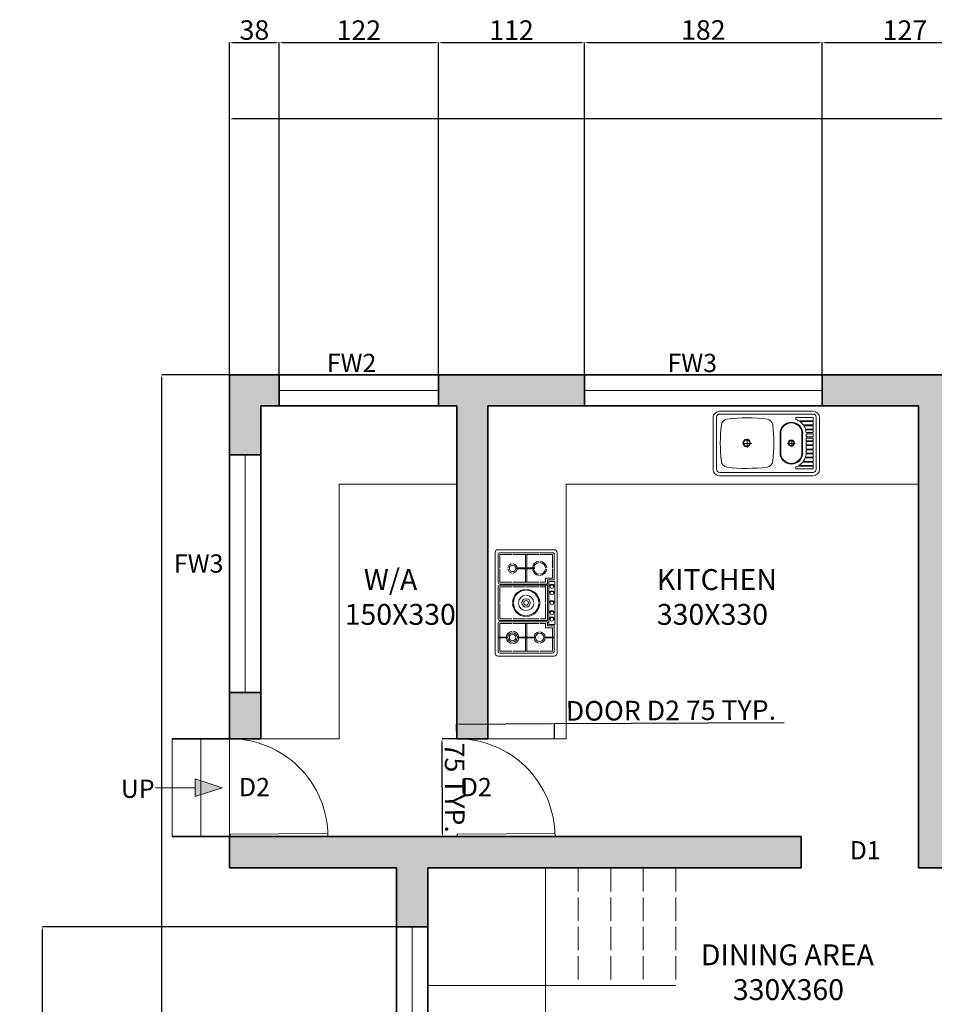
# Model space of a CAD drawing. Units: centimetres. Extents: x 2449 to 7478, y 778 to 2486.
# Tile 8 of 9: x 5994 to 6695, y 1732 to 2486. Entities that reach past the tile are written whole.
import ezdxf

# ---------------------------------------------------------------- set-up
doc = ezdxf.new("R2010")
doc.units = ezdxf.units.CM
doc.linetypes.add('ACAD_ISO02W100', pattern=[15, 12, -3])
for name, color, linetype, lineweight in [('A-ANNO-DIMS', 2, 'Continuous', 18), ('A-ANNO-SYMB', 8, 'Continuous', 18), ('A-ANNO-TEXT', 7, 'Continuous', 18), ('A-AREA-IDEN', 7, 'Continuous', 18), ('A-DOOR', 4, 'Continuous', 18), ('A-EQPM', 8, 'Continuous', 18), ('A-FLOR-CASE', 8, 'Continuous', 18), ('A-FLOR-FIXT', 8, 'Continuous', 18), ('A-FLOR-STRS', 7, 'Continuous', 18), ('A-FLOR-STRS-OVHD', 7, 'ACAD_ISO02W100', 13), ('A-WALL', 7, 'Continuous', 35), ('A-WALL-PATT', 7, 'Continuous', 13), ('Win', 1, 'Continuous', 18)]:
    doc.layers.add(name, color=color, linetype=linetype, lineweight=lineweight)
doc.styles.get("Standard").update_dxf_attribs({"font": 'arial.ttf'})
doc.dimstyles.new('ISO-25', dxfattribs={"dimtxt": 15, "dimasz": 2.5, "dimexe": 0, "dimexo": 0, "dimgap": 0, "dimtad": 1, "dimtxsty": 'Standard', "dimcen": 2.5, "dimadec": 0, "dimazin": 0, "dimtfac": 1, "dimtmove": 0, "dimatfit": 3, "dimfxl": 1, "dimarcsym": 0})

# ---------------------------------------------------------------- blocks, each defined once
blk = doc.blocks.new('sink 1')
for points in [[(-7.34, 1.48), (-7.34, 22.73)], [(-6.56, 1.48), (-6.56, 22.73)], [(5.86, 24.22), (-5.86, 24.22)], [(6.01, 23.43), (-5.86, 23.43)], [(6.72, 1.48), (6.72, 22.73)], [(7.34, 1.48), (7.34, 22.73)], [(1.09, 16.48), (-0.94, 16.48)], [(0, 15.39), (0, 17.42)], [(-2.09, 8.99), (2.28, 8.99)], [(-2.09, 8.84), (2.28, 8.84)], [(0, 5.55), (0, 7.26)], [(-5.78, 5.39), (-5.78, 5.39)], [(-5.31, 5.39), (-5.31, 5.39)], [(-5.16, 4.92), (-5.16, 4.92)], [(-5, 1.48), (-5, 4.69)], [(0.78, 6.33), (-0.78, 6.33)], [(5.16, 4.92), (5.16, 4.92)], [(5.94, 5.39), (5.94, 5.39)], [(-5, 1.48), (-4.22, 1.48), (-4.22, 3.83)], [(-4.84, 4.45), (-4.84, 4.45)], [(-4.22, 3.83), (-4.22, 3.83)], [(-4.06, 1.48), (-4.06, 3.69)], [(-4.06, 1.48), (-3.28, 1.48), (-3.28, 3.27)], [(-3.91, 3.52), (-3.91, 3.52)], [(-3.28, 3.2), (-3.28, 3.2)], [(-3.12, 3.2), (-3.12, 3.2)], [(-2.34, 3.05), (-2.34, 3.05)], [(-2.19, 3.05), (-2.19, 3.05)], [(-2.09, 3.99), (2.28, 3.99)], [(-2.09, 3.84), (2.28, 3.84)], [(-1.41, 3.05), (-1.41, 3.05)], [(-1.25, 3.05), (-1.25, 3.05)], [(-0.47, 1.48), (-1.25, 1.48), (-1.25, 3.05), (-0.47, 3.05)], [(-0.62, 3.05), (-0.62, 3.05)], [(-0.47, 1.48), (-0.47, 3.05)], [(-0.31, 3.05), (-0.31, 3.05)], [(0.47, 1.48), (-0.31, 1.48), (-0.31, 3.05), (0.47, 3.05)], [(0.31, 3.05), (0.31, 3.05)], [(0.47, 1.48), (0.47, 3.05)], [(0.62, 3.05), (0.62, 3.05)], [(1.25, 3.05), (1.25, 3.05)], [(1.56, 3.05), (1.56, 3.05)], [(2.19, 3.05), (2.19, 3.05)], [(2.5, 3.05), (2.5, 3.05)], [(3.12, 3.2), (3.12, 3.2)], [(3.28, 1.48), (4.06, 1.48), (4.06, 3.57)], [(3.28, 1.48), (3.28, 3.2)], [(3.44, 3.2), (3.44, 3.2)], [(4.06, 3.52), (4.06, 3.52)], [(4.22, 1.48), (4.22, 3.67)], [(4.37, 3.83), (4.37, 3.83)], [(5, 4.45), (5, 4.45)], [(6.01, 0.78), (-5.86, 0.78)], [(5.86, 0), (-5.86, 0)], [(-5.78, 1.48), (-5.78, 1.48)], [(-5.16, 1.48), (-5.16, 1.48)], [(-4.84, 1.48), (-4.84, 1.48)], [(-4.22, 1.48), (-4.22, 1.48)], [(-3.91, 1.48), (-3.91, 1.48)], [(-3.28, 1.48), (-3.28, 1.48)], [(-3.12, 1.48), (-3.12, 1.48)], [(-2.34, 1.48), (-2.34, 1.48)], [(-2.19, 1.48), (-2.19, 1.48)], [(-1.41, 1.48), (-1.41, 1.48)], [(-1.25, 1.48), (-1.25, 1.48)], [(-0.62, 1.48), (-0.62, 1.48)], [(-0.31, 1.48), (-0.31, 1.48)], [(0.31, 1.48), (0.31, 1.48)], [(0.62, 1.48), (0.62, 1.48)], [(1.25, 1.48), (1.25, 1.48)], [(1.56, 1.48), (1.56, 1.48)], [(2.19, 1.48), (2.19, 1.48)], [(2.5, 1.48), (2.5, 1.48)], [(3.12, 1.48), (3.12, 1.48)], [(3.44, 1.48), (3.44, 1.48)], [(4.06, 1.48), (4.06, 1.48)], [(4.37, 1.48), (4.37, 1.48)], [(5, 1.48), (5, 1.48)], [(5.16, 1.48), (5.16, 1.48)], [(5.94, 1.48), (5.94, 1.48)]]:
    blk.add_lwpolyline(points)
for points in [[(-5.16, 4.92), (-5.16, 1.48), (-5.78, 1.48), (-5.78, 5.39), (-5.31, 5.39, -0.068511), (-5.16, 4.92)], [(5.16, 4.92, 0.248301), (5.47, 5.39), (5.94, 5.39), (5.94, 1.48), (5.16, 1.48), (5.16, 4.92)], [(4.06, 3.57, -0.061679), (3.32, 3.22)], [(4.22, 1.48), (5, 1.48), (5, 4.45, -0.083542), (4.22, 3.67, -0.083542)]]:
    blk.add_lwpolyline(points, format="xyb")
for points in [[(-3.12, 3.22), (-3.12, 1.48), (-2.34, 1.48), (-2.34, 3.05, -0.06228)], [(2.5, 3.05), (2.5, 1.48), (3.12, 1.48), (3.12, 3.2, -0.050256)]]:
    blk.add_lwpolyline(points, format="xyb", close=True)
for points in [[(-2.19, 3.05), (-1.41, 3.05), (-1.41, 1.48), (-2.19, 1.48)], [(0.62, 3.05), (1.25, 3.05), (1.25, 1.48), (0.62, 1.48)], [(2.19, 1.48), (2.19, 3.05), (1.56, 3.05), (1.56, 1.48)]]:
    blk.add_lwpolyline(points, close=True)
for centre, radius in [((0.09, 16.57), 0.859), ((0.09, 16.57), 0.703), ((0.09, 6.41), 0.703), ((0.09, 6.41), 0.547)]:
    blk.add_circle(centre, radius)
for centre, radius, start, end in [((-5.86, 22.73), 1.48, 90, 180), ((-5.86, 22.73), 0.703, 90, 180), ((0.09, -12.65), 35.23, 83.2159, 96.7841), ((5.86, 22.73), 1.48, 360, 90), ((6.01, 22.73), 0.703, 0, 90), ((30.19, 16.56), 35.85, 172.7947, 187.4213), ((-3.87, 20.82), 1.53, 97.3256, 171.1849), ((4.06, 20.82), 1.53, 8.8151, 82.6744), ((-30, 16.56), 35.85, 352.5787, 7.2053), ((-3.89, 12.12), 1.48, 187.4212, 263.2159), ((4.08, 12.12), 1.48, 276.7841, 352.5788), ((-2.1, 6.41), 2.58, 90, 270), ((0.09, 45.63), 35.23, 263.2159, 276.7841), ((2.28, 6.41), 2.58, 270, 90), ((-2.1, 6.41), 2.42, 90, 270), ((2.28, 6.41), 2.42, 270, 90), ((-2.15, 6.48), 3.36, 212.1095, 232.0862), ((-2.1, 6.41), 3.36, 234.156, 249.3275), ((2.14, 6.36), 3.36, 289.8633, 290.5971), ((-5.86, 1.48), 1.48, 180, 270), ((-5.86, 1.48), 0.703, 180, 270), ((5.86, 1.48), 1.48, 270, 0), ((6.01, 1.48), 0.703, 270, 360)]:
    blk.add_arc(centre, radius, start, end)
blk = doc.blocks.new('STOVE')
for p, q in [((11.85, 19.7), (11.55, 19.7)), ((11.55, 16.92), (11.55, 19.7)), ((11.85, 16.92), (11.55, 16.92)), ((11.85, 16.92), (11.85, 19.7)), ((-11.85, 13.73), (-11.85, 7.62)), ((-11.85, 13.73), (-11.55, 13.73)), ((-11.55, 13.73), (-11.55, 7.62)), ((-11.85, 10.75), (-16.4, 10.75)), ((-11.85, 10.25), (-16.4, 10.25)), ((-7, 10.75), (-11.55, 10.75)), ((-7, 10.25), (-11.55, 10.25)), ((7, 10.75), (11.55, 10.75)), ((7, 10.25), (11.55, 10.25)), ((11.85, 13.23), (11.55, 13.23)), ((11.55, 13.23), (11.55, 7.57)), ((11.85, 13.23), (11.85, 7.57)), ((11.85, 10.75), (16.4, 10.75)), ((11.85, 10.25), (16.4, 10.25)), ((-11.85, 7.62), (-11.55, 7.62)), ((11.85, 7.57), (11.55, 7.57)), ((-7, 3.9), (-8.4, 3.9)), ((-5.4, 3.9), (-6, 3.9)), ((-5.4, 3.9), (-0.15, 3.9)), ((0.15, 3.9), (5.4, 3.9)), ((7, 3.9), (8.4, 3.9)), ((8.4, 3.9), (8.4, 1.6)), ((11.85, 4.28), (11.55, 4.28)), ((11.55, 4.28), (11.55, 1.3)), ((11.85, 4.28), (11.85, 1.3)), ((-7.8, 3.3), (-7.8, 1)), ((-6.4, 3.3), (-7.8, 3.3)), ((7.3, 2.8), (-7.3, 2.8)), ((-7.3, 2.8), (-7.3, 0.8)), ((7.3, 0.8), (-7.3, 0.8)), ((6.4, 3.3), (7.8, 3.3)), ((7.3, 2.8), (7.3, 0.8)), ((7.8, 3.3), (7.8, 1)), ((11.85, 1.3), (11.55, 1.3))]:
    blk.add_line(p, q)
for points in [[(-17, 21), (17, 21, -0.414214), (18, 20), (18, 1, -0.414214), (17, 0), (-17, 0, -0.414214), (-18, 1), (-18, 20, -0.414214)], [(6, 3.3), (-6, 3.3), (-6, 19.4, -0.414214), (-5.4, 20), (5.4, 20, -0.414214), (6, 19.4)]]:
    blk.add_lwpolyline(points, format="xyb", close=True)
for points in [[(-7.8, 1), (-16.4, 1, -0.414214), (-17, 1.6), (-17, 19.4, -0.414214), (-16.4, 20), (-7, 20, -0.414214), (-6.4, 19.4), (-6.4, 3.3)], [(6.4, 19.4, -0.414214), (7, 20), (16.4, 20, -0.414214), (17, 19.4), (17, 1.6, -0.414214), (16.4, 1), (7.8, 1)]]:
    blk.add_lwpolyline(points, format="xyb")
for points in [[(-16.4, 15.22), (-16.4, 19.4), (-11.85, 19.4)], [(-11.55, 19.4), (-7, 19.4), (-7, 15.22)], [(-5.4, 15.22), (-5.4, 19.4), (-0.15, 19.4)], [(0.15, 19.4), (5.4, 19.4), (5.4, 15.22)], [(6.4, 3.3), (6.4, 19.4)], [(7, 15.22), (7, 19.4), (11.55, 19.4)], [(11.85, 19.4), (16.4, 19.4), (16.4, 15.22)], [(-16.4, 6.08), (-16.4, 14.92)], [(-7, 14.92), (-7, 6.08)], [(-5.4, 10.65), (-5.4, 14.92)], [(5.4, 14.92), (5.4, 10.65)], [(7, 6.08), (7, 14.92)], [(16.4, 14.92), (16.4, 6.08)], [(-5.4, 6.08), (-5.4, 10.35)], [(5.4, 10.35), (5.4, 6.08)], [(-11.85, 1.6), (-16.4, 1.6), (-16.4, 5.77)], [(-8.4, 3.9), (-8.4, 1.6), (-11.55, 1.6)], [(-7, 5.77), (-7, 3.9)], [(-5.4, 3.9), (-5.4, 5.77)], [(5.4, 5.77), (5.4, 3.9)], [(7, 3.9), (7, 5.77)], [(16.4, 5.77), (16.4, 1.6), (11.85, 1.6)], [(11.55, 1.6), (8.4, 1.6)]]:
    blk.add_lwpolyline(points)
for centre, radius in [((-11.7, 15.07), 1.1), ((11.7, 15.07), 1.6), ((11.7, 15.07), 1.1), ((0, 10.5), 1.4), ((0, 10.5), 0.8), ((11.7, 5.93), 1.4), ((-5.49, 1.8), 0.6), ((-3.3, 1.8), 0.6), ((0, 1.8), 0.6), ((3.39, 1.8), 0.6), ((5.57, 1.8), 0.6)]:
    blk.add_circle(centre, radius)
for centre, radius, start, end in [((11.7, 15.07), 2.1, 94.096, 175.904), ((11.7, 15.07), 2.1, 4.096, 85.904), ((-11.7, 15.07), 1.6, 95.3794, 174.6206), ((-11.7, 15.07), 1.6, 185.3794, 264.6206), ((-11.7, 15.07), 1.6, 5.3794, 84.6206), ((-11.7, 15.07), 1.6, 275.3794, 354.6206), ((0, 10.5), 4.6, 91.8687, 178.1313), ((0, 10.5), 4.3, 91.9991, 178.0009), ((0, 10.5), 4.6, 1.8687, 88.1313), ((0, 10.5), 4.3, 1.9991, 88.0009), ((11.7, 15.07), 2.1, 184.096, 265.904), ((11.7, 15.07), 2.1, 274.096, 355.904), ((0, 10.5), 4.6, 181.8687, 268.1313), ((0, 10.5), 4.3, 181.9991, 268.0009), ((0, 10.5), 2.6, 93.3074, 176.6926), ((0, 10.5), 2.6, 183.3074, 266.6926), ((0, 10.5), 2.6, 3.3074, 86.6926), ((0, 10.5), 4.6, 271.8687, 358.1313), ((0, 10.5), 4.3, 271.9991, 358.0009), ((0, 10.5), 2.6, 273.3074, 356.6926), ((-11.7, 5.93), 2.4, 93.5833, 176.4167), ((-11.7, 5.93), 2, 94.3012, 175.6988), ((-11.7, 5.93), 2.4, 3.5833, 86.4167), ((-11.7, 5.93), 2, 4.3012, 85.6988), ((11.7, 5.93), 1.9, 94.5281, 175.4719), ((11.7, 5.93), 1.9, 4.5281, 85.4719), ((-11.7, 5.93), 2.4, 183.5833, 266.4167), ((-11.7, 5.93), 2, 184.3012, 265.6988), ((-11.7, 5.93), 2.4, 273.5833, 356.4167), ((-11.7, 5.93), 2, 274.3012, 355.6988), ((11.7, 5.93), 1.9, 184.5281, 265.4719), ((11.7, 5.93), 1.9, 274.5281, 355.4719), ((-5.49, 1.8), 0.846, 89.9979, 270), ((-3.3, 1.8), 0.846, 89.9979, 270), ((0, 1.8), 0.846, 89.9979, 270), ((3.39, 1.8), 0.846, 89.9979, 270), ((5.57, 1.8), 0.846, 89.9979, 270)]:
    blk.add_arc(centre, radius, start, end)
blk = doc.blocks.new('3')
for p, q in [((5936.31, 1821.57), (5936.31, 1746.57)), ((5938.31, 1821.57), (5938.31, 1746.57)), ((5938.31, 1746.57), (5936.31, 1746.57))]:
    blk.add_line(p, q)
blk.add_arc((5936.31, 1746.57), 75, 0, 90)
blk = doc.blocks.new('*D63')
at = {"layer": 'A-ANNO-DIMS', "color": 0, "lineweight": -2, "transparency": 16777216}
for p, q in [((6155.01, 2214.34), (6155.01, 2410.3)), ((7386.51, 2410.3), (6157.51, 2410.3)), ((7389.01, 2382.34), (7389.01, 2410.3))]:
    blk.add_line(p, q, dxfattribs=at)
at = {"layer": 'A-ANNO-DIMS', "color": 0, "transparency": 16777216}
for points in [[(6157.51, 2410.71), (6157.51, 2409.88), (6155.01, 2410.3)], [(7386.51, 2410.71), (7386.51, 2409.88), (7389.01, 2410.3)]]:
    blk.add_solid(points, dxfattribs=at)
at = {"layer": 'Defpoints', "color": 0, "transparency": 16777216}
for p in [(6155.01, 2410.3), (7389.01, 2382.34), (6155.01, 2214.34)]:
    blk.add_point(p, dxfattribs=at)
at = {"layer": 'A-ANNO-DIMS', "color": 0, "transparency": 16777216, "insert": (6772.01, 2417.96), "char_height": 15, "attachment_point": 5}
blk.add_mtext('1234', dxfattribs=at)
blk = doc.blocks.new('*D66')
at = {"layer": 'A-ANNO-DIMS', "color": 0, "lineweight": -2, "transparency": 16777216}
for p, q in [((6155.01, 2214.34), (6103.02, 2214.34)), ((6103.02, 1070.84), (6103.02, 2211.84)), ((6283.01, 1068.34), (6103.02, 1068.34))]:
    blk.add_line(p, q, dxfattribs=at)
at = {"layer": 'A-ANNO-DIMS', "color": 0, "transparency": 16777216}
for points in [[(6102.61, 2211.84), (6103.44, 2211.84), (6103.02, 2214.34)], [(6102.61, 1070.84), (6103.44, 1070.84), (6103.02, 1068.34)]]:
    blk.add_solid(points, dxfattribs=at)
at = {"layer": 'Defpoints', "color": 0, "transparency": 16777216}
for p in [(6103.02, 2214.34), (6155.01, 2214.34), (6283.01, 1068.34)]:
    blk.add_point(p, dxfattribs=at)
at = {"layer": 'A-ANNO-DIMS', "color": 0, "transparency": 16777216, "insert": (6095.36, 1641.34), "char_height": 15, "attachment_point": 5, "rotation": 90}
blk.add_mtext('1146', dxfattribs=at)
blk = doc.blocks.new('COUNTER-KITCHEN')
for p, q in [((0, 0), (270, 0)), ((0, 0), (0, -195)), ((0, -195), (-60, -195))]:
    blk.add_line(p, q)
blk = doc.blocks.new('COUNTER-UTILITY')
for p, q in [((0, 0), (90, 0)), ((0, 0), (0, -195)), ((-60, -195), (0, -195))]:
    blk.add_line(p, q)
blk = doc.blocks.new('ARROW-ENTRY-UP')
at = {"transparency": 33554687}
h = blk.add_hatch(color=256, dxfattribs=at)
h.dxf.hatch_style = 1
h.paths.add_polyline_path([(-6.84, 30.34), (6.84, 30.34), (0, 51.25)])
blk.add_line((0, 30.34), (0, 0))
blk.add_lwpolyline([(0, 51.25), (-6.84, 30.34), (6.84, 30.34)], close=True)
blk = doc.blocks.new('*D76')
at = {"layer": 'A-ANNO-DIMS', "color": 0, "lineweight": -2, "transparency": 16777216}
for p, q in [((6329.01, 1935.34), (6328.95, 1946.59)), ((6331.45, 1946.6), (6401.45, 1946.93)), ((6403.95, 1946.94), (6580.01, 1947.78)), ((6404.01, 1935.69), (6403.95, 1946.94))]:
    blk.add_line(p, q, dxfattribs=at)
at = {"layer": 'A-ANNO-DIMS', "color": 0, "transparency": 16777216}
for points in [[(6331.45, 1947.02), (6331.45, 1946.18), (6328.95, 1946.59)], [(6401.45, 1947.35), (6401.45, 1946.52), (6403.95, 1946.94)]]:
    blk.add_solid(points, dxfattribs=at)
at = {"layer": 'Defpoints', "color": 0, "transparency": 16777216}
for p in [(6403.95, 1946.94), (6329.01, 1935.34), (6404.01, 1935.69)]:
    blk.add_point(p, dxfattribs=at)
at = {"layer": 'A-ANNO-DIMS', "color": 0, "transparency": 16777216, "insert": (6493.2, 1955.13), "char_height": 15, "attachment_point": 5, "rotation": 0.27085}
blk.add_mtext('DOOR D2 75 TYP.', dxfattribs=at)
blk = doc.blocks.new('*D77')
at = {"layer": 'A-ANNO-DIMS', "color": 0, "lineweight": -2, "transparency": 16777216}
for p, q in [((6329.01, 1935.34), (6317.76, 1935.29)), ((6318.1, 1862.79), (6317.77, 1932.79)), ((6329.36, 1860.34), (6318.11, 1860.29))]:
    blk.add_line(p, q, dxfattribs=at)
at = {"layer": 'A-ANNO-DIMS', "color": 0, "transparency": 16777216}
for points in [[(6318.18, 1932.79), (6317.35, 1932.78), (6317.76, 1935.29)], [(6318.52, 1862.79), (6317.68, 1862.79), (6318.11, 1860.29)]]:
    blk.add_solid(points, dxfattribs=at)
at = {"layer": 'Defpoints', "color": 0, "transparency": 16777216}
for p in [(6317.76, 1935.29), (6329.01, 1935.34), (6329.36, 1860.34)]:
    blk.add_point(p, dxfattribs=at)
at = {"layer": 'A-ANNO-DIMS', "color": 0, "transparency": 16777216, "insert": (6325.56, 1897.82), "char_height": 15, "attachment_point": 5, "rotation": 270.27085}
blk.add_mtext('75 TYP.', dxfattribs=at)
blk = doc.blocks.new('*D105')
at = {"layer": 'A-ANNO-DIMS', "color": 0, "lineweight": -2, "transparency": 16777216}
for p, q in [((6155.01, 2214.34), (6155.01, 2468.84)), ((6157.51, 2468.84), (6190.51, 2468.84)), ((6193.01, 2214.34), (6193.01, 2468.84))]:
    blk.add_line(p, q, dxfattribs=at)
at = {"layer": 'A-ANNO-DIMS', "color": 0, "transparency": 16777216}
for points in [[(6157.51, 2469.26), (6157.51, 2468.42), (6155.01, 2468.84)], [(6190.51, 2469.26), (6190.51, 2468.42), (6193.01, 2468.84)]]:
    blk.add_solid(points, dxfattribs=at)
at = {"layer": 'Defpoints', "color": 0, "transparency": 16777216}
for p in [(6193.01, 2468.84), (6155.01, 2214.34), (6193.01, 2214.34)]:
    blk.add_point(p, dxfattribs=at)
at = {"layer": 'A-ANNO-DIMS', "color": 0, "transparency": 16777216, "insert": (6174.01, 2476.5), "char_height": 15, "attachment_point": 5}
blk.add_mtext('38', dxfattribs=at)
blk = doc.blocks.new('*D106')
at = {"layer": 'A-ANNO-DIMS', "color": 0, "lineweight": -2, "transparency": 16777216}
for p, q in [((6193.01, 2214.34), (6193.01, 2468.84)), ((6195.51, 2468.84), (6312.51, 2468.84)), ((6315.01, 2214.34), (6315.01, 2468.84))]:
    blk.add_line(p, q, dxfattribs=at)
at = {"layer": 'A-ANNO-DIMS', "color": 0, "transparency": 16777216}
for points in [[(6195.51, 2469.26), (6195.51, 2468.42), (6193.01, 2468.84)], [(6312.51, 2469.26), (6312.51, 2468.42), (6315.01, 2468.84)]]:
    blk.add_solid(points, dxfattribs=at)
at = {"layer": 'Defpoints', "color": 0, "transparency": 16777216}
for p in [(6315.01, 2468.84), (6193.01, 2214.34), (6315.01, 2214.34)]:
    blk.add_point(p, dxfattribs=at)
at = {"layer": 'A-ANNO-DIMS', "color": 0, "transparency": 16777216, "insert": (6254.01, 2476.37), "char_height": 15, "attachment_point": 5}
blk.add_mtext('122', dxfattribs=at)
blk = doc.blocks.new('*D107')
at = {"layer": 'A-ANNO-DIMS', "color": 0, "lineweight": -2, "transparency": 16777216}
for p, q in [((6315.01, 2214.34), (6315.01, 2468.84)), ((6317.51, 2468.84), (6424.51, 2468.84)), ((6427.01, 2214.34), (6427.01, 2468.84))]:
    blk.add_line(p, q, dxfattribs=at)
at = {"layer": 'A-ANNO-DIMS', "color": 0, "transparency": 16777216}
for points in [[(6317.51, 2469.26), (6317.51, 2468.42), (6315.01, 2468.84)], [(6424.51, 2469.26), (6424.51, 2468.42), (6427.01, 2468.84)]]:
    blk.add_solid(points, dxfattribs=at)
at = {"layer": 'Defpoints', "color": 0, "transparency": 16777216}
for p in [(6427.01, 2468.84), (6315.01, 2214.34), (6427.01, 2214.34)]:
    blk.add_point(p, dxfattribs=at)
at = {"layer": 'A-ANNO-DIMS', "color": 0, "transparency": 16777216, "insert": (6371.01, 2476.37), "char_height": 15, "attachment_point": 5}
blk.add_mtext('112', dxfattribs=at)
blk = doc.blocks.new('*D108')
at = {"layer": 'A-ANNO-DIMS', "color": 0, "lineweight": -2, "transparency": 16777216}
for p, q in [((6427.01, 2214.34), (6427.01, 2468.84)), ((6429.51, 2468.84), (6606.51, 2468.84)), ((6609.01, 2214.34), (6609.01, 2468.84))]:
    blk.add_line(p, q, dxfattribs=at)
at = {"layer": 'A-ANNO-DIMS', "color": 0, "transparency": 16777216}
for points in [[(6429.51, 2469.26), (6429.51, 2468.42), (6427.01, 2468.84)], [(6606.51, 2469.26), (6606.51, 2468.42), (6609.01, 2468.84)]]:
    blk.add_solid(points, dxfattribs=at)
at = {"layer": 'Defpoints', "color": 0, "transparency": 16777216}
for p in [(6609.01, 2468.84), (6427.01, 2214.34), (6609.01, 2214.34)]:
    blk.add_point(p, dxfattribs=at)
at = {"layer": 'A-ANNO-DIMS', "color": 0, "transparency": 16777216, "insert": (6518.01, 2476.5), "char_height": 15, "attachment_point": 5}
blk.add_mtext('182', dxfattribs=at)
blk = doc.blocks.new('*D109')
at = {"layer": 'A-ANNO-DIMS', "color": 0, "lineweight": -2, "transparency": 16777216}
for p, q in [((6609.01, 2214.34), (6609.01, 2468.84)), ((6611.51, 2468.84), (6733.51, 2468.84)), ((6736.01, 2214.34), (6736.01, 2468.84))]:
    blk.add_line(p, q, dxfattribs=at)
at = {"layer": 'A-ANNO-DIMS', "color": 0, "transparency": 16777216}
for points in [[(6611.51, 2469.26), (6611.51, 2468.42), (6609.01, 2468.84)], [(6733.51, 2469.26), (6733.51, 2468.42), (6736.01, 2468.84)]]:
    blk.add_solid(points, dxfattribs=at)
at = {"layer": 'Defpoints', "color": 0, "transparency": 16777216}
for p in [(6736.01, 2468.84), (6609.01, 2214.34), (6736.01, 2214.34)]:
    blk.add_point(p, dxfattribs=at)
at = {"layer": 'A-ANNO-DIMS', "color": 0, "transparency": 16777216, "insert": (6672.51, 2476.37), "char_height": 15, "attachment_point": 5}
blk.add_mtext('127', dxfattribs=at)
blk = doc.blocks.new('*D115')
at = {"layer": 'A-ANNO-DIMS', "color": 0, "lineweight": -2, "transparency": 16777216}
for p, q in [((6283.01, 1791.34), (6011.65, 1791.34)), ((6011.65, 1553.84), (6011.65, 1788.84)), ((6283.01, 1551.34), (6011.65, 1551.34))]:
    blk.add_line(p, q, dxfattribs=at)
at = {"layer": 'A-ANNO-DIMS', "color": 0, "transparency": 16777216}
for points in [[(6011.23, 1788.84), (6012.07, 1788.84), (6011.65, 1791.34)], [(6011.23, 1553.84), (6012.07, 1553.84), (6011.65, 1551.34)]]:
    blk.add_solid(points, dxfattribs=at)
at = {"layer": 'Defpoints', "color": 0, "transparency": 16777216}
for p in [(6011.65, 1791.34), (6283.01, 1791.34), (6283.01, 1551.34)]:
    blk.add_point(p, dxfattribs=at)
at = {"layer": 'A-ANNO-DIMS', "color": 0, "transparency": 16777216, "insert": (6003.99, 1671.34), "char_height": 15, "attachment_point": 5, "rotation": 90}
blk.add_mtext('240', dxfattribs=at)

msp = doc.modelspace()

# ---------------------------------------------------------------- hatches: boundary and pattern name
at = {"layer": 'A-WALL-PATT'}
h = msp.add_hatch(color=256, dxfattribs=at)
h.dxf.hatch_style = 1
h.paths.add_polyline_path([(6637.006, 1092.34), (6563.006, 1092.34), (6563.006, 1068.34), (6661.006, 1068.34), (6661.006, 1476.34), (6637.006, 1476.34)])
h.paths.add_polyline_path([(6283.006, 1167.34), (6307.006, 1167.34), (6307.006, 1377.34), (6283.006, 1377.34)])
h.paths.add_polyline_path([(6381.006, 1068.34), (6381.006, 1092.34), (6307.006, 1092.34), (6307.006, 1112.34), (6283.006, 1112.34), (6283.006, 1068.34)])
h.paths.add_polyline_path([(6307.006, 1551.34), (6283.006, 1551.34), (6283.006, 1432.34), (6307.006, 1432.34), (6307.006, 1452.34), (6547.006, 1452.34), (6547.006, 1476.34), (6307.006, 1476.34)])
h.paths.add_polyline_path([(7011.006, 1654.34), (7011.006, 1266.34), (6982.006, 1266.34), (6982.006, 1242.34), (7035.006, 1242.34), (7035.006, 1404.34), (7059.006, 1404.34), (7059.006, 1428.34), (7035.006, 1428.34), (7035.006, 1678.34), (6837.006, 1678.34), (6837.006, 1654.34)])
h.paths.add_polyline_path([(6800.006, 1266.34), (6771.006, 1266.34), (6771.006, 1242.34), (6800.006, 1242.34)])
h.paths.add_polyline_path([(7389.006, 1506.339), (7365.006, 1506.339), (7365.006, 1428.34), (7341.006, 1428.34), (7341.006, 1404.34), (7389.006, 1404.34)])
h.paths.add_polyline_path([(7286.006, 1404.34), (7286.006, 1428.34), (7114.006, 1428.34), (7114.006, 1404.34)])
h.paths.add_polyline_path([(7365.006, 1688.339), (7389.006, 1688.339), (7389.006, 1826.34), (7365.006, 1826.34), (7365.006, 1792.34), (7224.006, 1792.34), (7224.006, 1768.34), (7365.006, 1768.34)])
h.paths.add_polyline_path([(7365.006, 1956.34), (7125.006, 1956.34), (7125.006, 1792.34), (7011.006, 1792.34), (7011.006, 1768.34), (7149.006, 1768.34), (7149.006, 1932.34), (7365.006, 1932.34), (7365.006, 1898.34), (7389.006, 1898.34), (7389.006, 2065.339), (7365.006, 2065.339)])
h.paths.add_polyline_path([(7365.006, 2358.34), (7365.006, 2247.339), (7389.006, 2247.339), (7389.006, 2382.34), (7341.006, 2382.34), (7341.006, 2358.34)])
h.paths.add_polyline_path([(7114.006, 2382.34), (7114.006, 2358.34), (7286.006, 2358.34), (7286.006, 2382.34)])
h.paths.add_polyline_path([(7035.006, 2358.34), (7059.006, 2358.34), (7059.006, 2382.34), (7011.006, 2382.34), (7011.006, 2214.34), (6972.006, 2214.34), (6972.006, 2190.34), (7011.006, 2190.34), (7011.006, 2065.34), (7035.006, 2065.34)])
h.paths.add_polyline_path([(6808.006, 2214.34), (6808.006, 2190.34), (6837.006, 2190.34), (6837.006, 1966.34), (7011.006, 1966.34), (7011.006, 1932.34), (7035.006, 1932.34), (7035.006, 1990.34), (6861.006, 1990.34), (6861.006, 2190.34), (6900.006, 2190.34), (6900.006, 2214.34)])
h.paths.add_polyline_path([(6707.006, 2190.34), (6736.006, 2190.34), (6736.006, 2214.34), (6609.006, 2214.34), (6609.006, 2190.34), (6683.006, 2190.34), (6683.006, 1836.34), (6707.006, 1836.34), (6707.006, 1966.34), (6762.006, 1966.34), (6762.006, 1990.34), (6707.006, 1990.34)])
h.paths.add_polyline_path([(6315.006, 2214.34), (6315.006, 2190.34), (6329.006, 2190.34), (6329.006, 1935.34), (6353.006, 1935.34), (6353.006, 2190.34), (6427.006, 2190.34), (6427.006, 2214.34)])
h.paths.add_polyline_path([(6155.006, 2152.839), (6179.006, 2152.839), (6179.006, 2190.34), (6193.006, 2190.34), (6193.006, 2214.34), (6155.006, 2214.34)])
h.paths.add_polyline_path([(6155.006, 1935.34), (6179.006, 1935.34), (6179.006, 1970.839), (6155.006, 1970.839)])
h.paths.add_polyline_path([(6283.006, 1836.34), (6283.006, 1791.34), (6307.006, 1791.34), (6307.006, 1836.34), (6593.006, 1836.34), (6593.006, 1860.34), (6155.006, 1860.34), (6155.006, 1836.34)])

# ---------------------------------------------------------------- linework, layer by layer
at = {"layer": 'A-FLOR-STRS'}
for p, q in [((6111.006, 1935.34), (6111.006, 1860.34)), ((6133.006, 1935.34), (6133.006, 1860.34)), ((6155.006, 1935.34), (6155.006, 1860.34)), ((6397.006, 1836.34), (6397.006, 1476.34)), ((6307.006, 1746.34), (6497.006, 1746.34))]:
    msp.add_line(p, q, dxfattribs=at)
at = {"layer": 'A-FLOR-STRS-OVHD', "ltscale": 1.5}
for p, q in [((6422.006, 1836.34), (6422.006, 1746.34)), ((6447.006, 1836.34), (6447.006, 1746.34)), ((6472.006, 1836.34), (6472.006, 1746.34)), ((6497.006, 1836.34), (6497.006, 1746.34))]:
    msp.add_line(p, q, dxfattribs=at)
at = {"layer": 'A-WALL'}
for p, q in [((6155.006, 2214.34), (7011.006, 2214.34)), ((6155.006, 2214.34), (6155.006, 1935.34)), ((6193.006, 2190.34), (6193.006, 2214.34)), ((6315.006, 2190.34), (6315.006, 2214.34)), ((6427.006, 2190.34), (6427.006, 2214.34)), ((6609.006, 2190.34), (6609.006, 2214.34)), ((6179.006, 2190.34), (6329.006, 2190.34)), ((6179.006, 2190.34), (6179.006, 1935.34)), ((6329.006, 2190.34), (6329.006, 1935.34)), ((6353.006, 2190.34), (6683.006, 2190.34)), ((6353.006, 2190.34), (6353.006, 1935.34)), ((6683.006, 2190.34), (6683.006, 1836.34)), ((6155.006, 2152.839), (6179.006, 2152.839)), ((6155.006, 1970.839), (6179.006, 1970.839)), ((6111.006, 1935.34), (6179.006, 1935.34)), ((6329.006, 1935.34), (6353.006, 1935.34)), ((6111.006, 1860.34), (6593.006, 1860.34)), ((6155.006, 1860.34), (6155.006, 1836.34)), ((6593.006, 1860.34), (6593.006, 1836.34)), ((6155.006, 1836.34), (6283.006, 1836.34)), ((6283.006, 1836.34), (6283.006, 1068.34)), ((6307.006, 1836.34), (6593.006, 1836.34)), ((6307.006, 1836.34), (6307.006, 1476.34)), ((6683.006, 1836.34), (6707.006, 1836.34)), ((6307.006, 1791.34), (6283.006, 1791.34))]:
    msp.add_line(p, q, dxfattribs=at)
at = {"layer": 'Win'}
for p, q in [((6193.006, 2202.34), (6315.006, 2202.34)), ((6427.006, 2202.34), (6609.006, 2202.34)), ((6167.006, 2152.839), (6167.006, 1970.839)), ((6295.006, 1791.34), (6295.006, 1551.34))]:
    msp.add_line(p, q, dxfattribs=at)

# ---------------------------------------------------------------- block references
at = {"layer": 'A-ANNO-SYMB', "rotation": 269.9999999999995}
msp.add_blockref('ARROW-ENTRY-UP', (6098.15, 1897.84), dxfattribs=at)
at = {"layer": 'A-DOOR', "xscale": -1, "rotation": 270.2708478329989}
for p in [(4436.875, -4084.159), (4610.875, -4084.159)]:
    msp.add_blockref('3', p, dxfattribs=at)
at = {"layer": 'A-EQPM', "xscale": -2.262184600755962, "yscale": 2.262184600755962, "zscale": 2.262184600755962, "rotation": 90}
msp.add_blockref('STOVE', (6405.961, 2039.449), dxfattribs=at)
at = {"layer": 'A-FLOR-CASE'}
for name, p in [('COUNTER-UTILITY', (6239.006, 2130.34)), ('COUNTER-KITCHEN', (6413.006, 2130.34))]:
    msp.add_blockref(name, p, dxfattribs=at)
at = {"layer": 'A-FLOR-FIXT', "xscale": 3.367959604697591, "yscale": 3.367959604697591, "zscale": 3.367959604697591, "rotation": 90}
msp.add_blockref('sink 1', (6607.053, 2161.57), dxfattribs=at)

# ---------------------------------------------------------------- texts
at = {"layer": 'A-ANNO-TEXT', "char_height": 14, "attachment_point": 1}
for s, insert in [('{\\fTimes New Roman|b0|i0|c0|p18;\\P   FW2}', (6216.68, 2253.652)), ('{\\fTimes New Roman|b0|i0|c0|p18;\\P   FW3}', (6477.755, 2253.652)), ('{\\fTimes New Roman|b0|i0|c0|p18;\\PFW3}', (6112.349, 2099.963)), ('{\\fTimes New Roman|b0|i0|c0|p18;\\PUP}', (6071.632, 1927.379)), ('{\\fTimes New Roman|b0|i0|c0|p18;\\PD2}', (6162.157, 1928.696)), ('{\\fTimes New Roman|b0|i0|c0|p18;\\PD2}', (6332.157, 1928.696)), ('{\\fTimes New Roman|b0|i0|c0|p18;\\PD1}', (6630.168, 1880.265))]:
    msp.add_mtext_dynamic_manual_height_columns(s, width=211.90348, gutter_width=12.5, heights=[0], dxfattribs=dict(at, insert=insert))
at = {"layer": 'A-AREA-IDEN', "char_height": 16, "attachment_point": 1}
for s, insert in [('{\\fTimes New Roman|b0|i0|c0|p18;\\P   W/A\\P150X330}', (6243.171, 2092)), ('{\\fTimes New Roman|b0|i0|c0|p18;\\PKITCHEN\\P330X330}', (6482.371, 2092)), ('{\\fTimes New Roman|b0|i0|c0|p18;\\P DINING AREA\\P      330X360}', (6511.288, 1804.477))]:
    msp.add_mtext_dynamic_manual_height_columns(s, width=211.90348, gutter_width=12.5, heights=[0], dxfattribs=dict(at, insert=insert))

# ---------------------------------------------------------------- dimensions: what is measured, and where the dimension line sits
at = {"layer": 'A-ANNO-DIMS'}
for base, p1, p2, override, picture, middle in [((6193.006, 2468.84), (6155.006, 2214.34), (6193.006, 2214.34), {"dimdec": 0, "dimlfac": 1, "dimrnd": 0, "dimzin": 0, "dimdsep": 46, "dimlunit": 2}, '*D105', (6174.006, 2476.503)), ((6315.006, 2468.84), (6193.006, 2214.34), (6315.006, 2214.34), {"dimdec": 0, "dimlfac": 1, "dimrnd": 0, "dimzin": 0, "dimdsep": 46, "dimlunit": 2}, '*D106', (6254.006, 2476.37)), ((6427.006, 2468.84), (6315.006, 2214.34), (6427.006, 2214.34), {"dimdec": 0, "dimlfac": 1, "dimrnd": 0, "dimzin": 0, "dimdsep": 46, "dimlunit": 2}, '*D107', (6371.006, 2476.37)), ((6609.006, 2468.84), (6427.006, 2214.34), (6609.006, 2214.34), {"dimdec": 0, "dimlfac": 1, "dimrnd": 0, "dimzin": 0, "dimdsep": 46, "dimlunit": 2}, '*D108', (6518.006, 2476.498)), ((6736.006, 2468.84), (6609.006, 2214.34), (6736.006, 2214.34), {"dimdec": 0, "dimlfac": 1, "dimrnd": 0, "dimzin": 0, "dimdsep": 46, "dimlunit": 2}, '*D109', (6672.506, 2476.37)), ((6155.006, 2410.295), (7389.006, 2382.34), (6155.006, 2214.34), {"dimclrd": 0, "dimclre": 0, "dimclrt": 0}, '*D63', (6772.006, 2417.959))]:
    dim = msp.add_linear_dim(base=base, p1=p1, p2=p2, dimstyle='ISO-25', override=override, dxfattribs=at)
    dim.commit()
    dim.dimension.update_dxf_attribs({"geometry": picture, "text_midpoint": middle})
for base, p1, p2, override, picture, middle in [((6103.023, 2214.34), (6283.006, 1068.34), (6155.006, 2214.34), {"dimclrd": 0, "dimclre": 0, "dimclrt": 0}, '*D66', (6095.365, 1641.34)), ((6011.65, 1791.34), (6283.006, 1551.34), (6283.006, 1791.34), {"dimdec": 0, "dimlfac": 1, "dimrnd": 0, "dimzin": 0, "dimdsep": 46, "dimlunit": 2}, '*D115', (6003.991, 1671.34))]:
    dim = msp.add_linear_dim(base=base, p1=p1, p2=p2, angle=90, dimstyle='ISO-25', override=override, dxfattribs=at)
    dim.commit()
    dim.dimension.update_dxf_attribs({"geometry": picture, "text_midpoint": middle})
for base, p1, p2, angle, text, picture, middle in [((6403.952, 1946.944), (6329.006, 1935.34), (6404.005, 1935.694), 0.270848, 'DOOR D2 <> TYP.', '*D76', (6493.196, 1955.127)), ((6317.756, 1935.287), (6329.361, 1860.341), (6329.006, 1935.34), 90.270848, '<> TYP.', '*D77', (6325.561, 1897.823))]:
    dim = msp.add_linear_dim(base=base, p1=p1, p2=p2, angle=angle, text=text, dimstyle='ISO-25', override={"dimdec": 0, "dimlfac": 1, "dimrnd": 0, "dimzin": 0, "dimdsep": 46, "dimlunit": 2}, dxfattribs=at)
    dim.commit()
    dim.dimension.update_dxf_attribs({"geometry": picture, "text_midpoint": middle})

doc.saveas('drawing.dxf')
